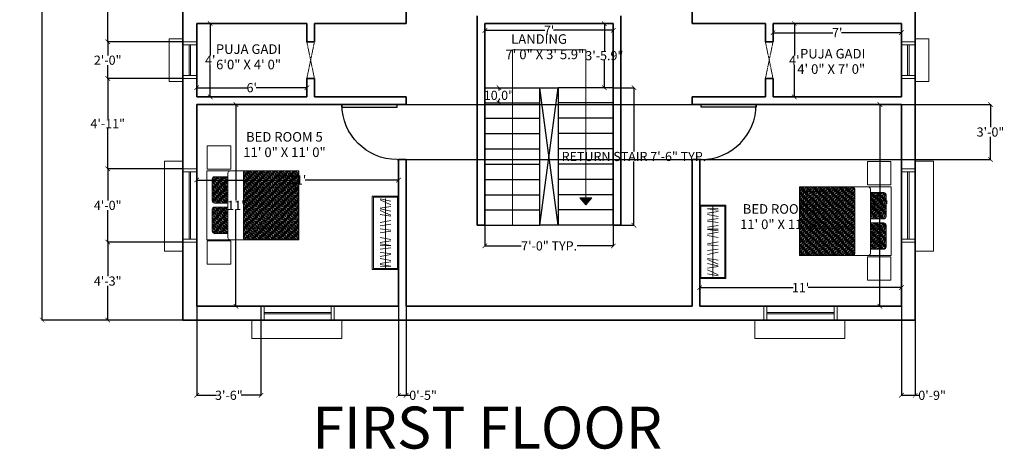
# Model space of a CAD drawing. Units: inches. Extents: x 844 to 2234, y 346 to 1084.
# Tile 47 of 93: x 1590 to 2234, y 351 to 632. Entities that reach past the tile are written whole.
import ezdxf

# ---------------------------------------------------------------- set-up
doc = ezdxf.new("R2010")
doc.units = ezdxf.units.IN
doc.header["$MEASUREMENT"] = 0
doc.linetypes.add('DASHED', pattern=[0.75, 0.5, -0.25])
for name, color, linetype, lineweight in [('A-ANNO-DIMS', 2, 'Continuous', 18), ('A-ANNO-SYMB', 7, 'Continuous', 18), ('A-ANNO-TEXT', 7, 'Continuous', 35), ('A-AREA-IDEN', 7, 'Continuous', 18), ('A-FLOR-STRS', 7, 'Continuous', 25), ('A-WALL', 7, 'Continuous', 35), ('A-WALL-OVHD', 7, 'DASHED', 18), ('beds', 130, 'Continuous', 18), ('doors', 170, 'Continuous', 25), ('furniture', 8, 'Continuous', 18), ('windows', 1, 'Continuous', 18)]:
    doc.layers.add(name, color=color, linetype=linetype, lineweight=lineweight)
doc.styles.get("Standard").update_dxf_attribs({"font": 'arial.ttf'})
doc.dimstyles.get("Standard").update_dxf_attribs({"dimtxt": 6, "dimasz": 3, "dimexe": 0.18, "dimexo": 0.0625, "dimgap": 0.09, "dimtad": 0, "dimtih": 1, "dimtoh": 1, "dimdec": 1, "dimzin": 0, "dimdsep": 46, "dimlunit": 3, "dimtxsty": 'Standard', "dimblk": 'ARCHTICK', "dimcen": 0.09, "dimadec": 0, "dimazin": 0, "dimtfac": 1, "dimtdec": 1, "dimtofl": 0, "dimtmove": 0, "dimatfit": 3, "dimfxl": 1, "dimtolj": 1, "dimtzin": 0, "dimarcsym": 0})
pattern_1 = [(135, (-1377.70473, -125.71507), (-0.070710678, -0.070710678), []), (135, (-1377.68705, -125.69739), (-0.070710678, -0.070710678), []), (45, (-1377.70473, -125.71507), (-0.070710678, 0.070710678), [-0.025, 0.025]), (45, (-1377.72241, -125.69739), (-0.070710678, 0.070710678), [-0.025, 0.025]), (45, (-1377.74009, -125.67972), (-0.070710678, 0.070710678), [0.025, -0.025]), (45, (-1377.75776, -125.66204), (-0.070710678, 0.070710678), [0.025, -0.025]), (135, (-1377.66938, -125.67972), (-0.070710678, -0.070710678), [0.025, -0.025]), (135, (-1377.6517, -125.66204), (-0.070710678, -0.070710678), [0.025, -0.025])]

# ---------------------------------------------------------------- blocks, each defined once
blk = doc.blocks.new('*U2')
for p, q in [((0, 0), (0, -6)), ((36, 0), (36, -6))]:
    blk.add_line(p, q)
blk.add_lwpolyline([(0, 0), (0, 36), (1.75, 36), (1.75, 0)], close=True)
blk.add_arc((0, 0), 36, 0, 90)
blk = doc.blocks.new('MAT-P10')
h = blk.add_hatch()
h.set_pattern_fill('BOX', color=256, scale=0.1, angle=45, style=0)
h.set_pattern_definition(pattern_1)
h.paths.add_polyline_path([(-0.157, 1.46), (0.417, 1.46), (0.417, 1.751, 0.414214), (0.367, 1.801), (-0.107, 1.801, 0.414214), (-0.157, 1.751)])
h.paths.add_polyline_path([(0.505, 1.46), (1.079, 1.46), (1.079, 1.751, 0.414214), (1.029, 1.801), (0.555, 1.801, 0.414214), (0.505, 1.751)])
h = blk.add_hatch()
h.set_pattern_fill('BOX', color=256, scale=0.1, angle=45, style=0)
h.set_pattern_definition(pattern_1)
edge = h.paths.add_edge_path()
edge.add_line((1.205, -0.085), (1.205, 1.062))
edge.add_ellipse((1.161, 1.063), major_axis=(0, 0.0568), ratio=0.776379, start_angle=270, end_angle=360)
edge.add_line((1.161, 1.119), (-0.251, 1.12))
edge.add_ellipse((-0.251, 1.063), major_axis=(0, 0.0568), ratio=0.776379, start_angle=0, end_angle=88.1396)
edge.add_line((-0.295, 1.064), (-0.295, -0.085))
edge.add_line((-0.295, -0.085), (1.205, -0.085))
for p, q in [((-0.251, 1.46), (1.161, 1.46)), ((-0.251, 1.12), (1.161, 1.119)), ((1.102, 0.406), (1.102, 0.057)), ((1.058, 0), (0.775, 0))]:
    blk.add_line(p, q)
for points in [[(-0.83, 1.909), (-0.319, 1.909), (-0.319, 1.398), (-0.83, 1.398)], [(1.205, -0.085), (-0.295, -0.085), (-0.295, 1.915), (1.205, 1.915)], [(1.244, 1.909), (1.755, 1.909), (1.755, 1.398), (1.244, 1.398)]]:
    blk.add_lwpolyline(points, close=True)
for points in [[(0.417, 1.46), (0.417, 1.751, 0.414214), (0.367, 1.801), (-0.107, 1.801, 0.414214), (-0.157, 1.751), (-0.157, 1.46)], [(1.079, 1.46), (1.079, 1.751, 0.414214), (1.029, 1.801), (0.555, 1.801, 0.414214), (0.505, 1.751), (0.505, 1.46)], [(0.37, 1.624), (0.37, 1.571, -0.414214), (0.32, 1.521), (0.111, 1.521)], [(1.012, 1.644), (1.012, 1.571, -0.414214), (0.962, 1.521), (0.753, 1.521)]]:
    blk.add_lwpolyline(points, format="xyb")
at = {"extrusion": (0, 0, -1)}
for centre, start_param, end_param in [((-0.251, 1.404), 4.712389, 6.283185), ((1.161, 1.404), 0, 1.570796), ((-0.251, 1.063), 4.712389, 6.283185), ((1.161, 1.063), 0, 1.570796), ((1.058, 0.057), 1.570796, 3.141593), ((1.058, 0.057), 1.570796, 3.141593)]:
    blk.add_ellipse(centre, major_axis=(0, 0.0568), ratio=0.776379, start_param=start_param, end_param=end_param, dxfattribs=at)
blk = doc.blocks.new('A$C7A17768A')
for p, q in [((-2.8, 0), (0, 0)), ((-2.8, -1), (-2.8, 0)), ((0, -1), (0, 0)), ((-2.76, -0.04), (-0.04, -0.04)), ((-2.76, -0.96), (-2.76, -0.04)), ((-2.617, -0.3), (-2.694, -0.7)), ((-2.66, -0.7), (-2.466, -0.3)), ((-2.403, -0.3), (-2.342, -0.7)), ((-2.229, -0.296), (-2.317, -0.696)), ((-2.074, -0.3), (-2.25, -0.7)), ((-2.096, -0.7), (-2.033, -0.3)), ((-1.875, -0.3), (-1.796, -0.7)), ((-1.732, -0.3), (-1.675, -0.7)), ((-1.555, -0.7), (-1.507, -0.3)), ((-1.467, -0.3), (-1.403, -0.7)), ((-1.227, -0.7), (-1.151, -0.3)), ((-1.098, -0.3), (-1.034, -0.7)), ((-0.98, -0.7), (-0.921, -0.3)), ((-0.908, -0.3), (-0.919, -0.7)), ((-0.834, -0.3), (-0.777, -0.7)), ((-0.657, -0.7), (-0.61, -0.3)), ((-0.57, -0.3), (-0.505, -0.7)), ((-0.429, -0.7), (-0.353, -0.3)), ((-0.301, -0.3), (-0.237, -0.7)), ((-0.192, -0.7), (-0.133, -0.3)), ((-0.12, -0.3), (-0.131, -0.7)), ((-0.04, -0.96), (-0.04, -0.04)), ((-0.04, -0.5), (-2.716, -0.5)), ((-2.8, -1), (0, -1)), ((-2.76, -0.96), (-0.04, -0.96))]:
    blk.add_line(p, q)
blk = doc.blocks.new('_ArchTick')
at = {"color": 0, "linetype": 'ByBlock', "const_width": 0.15}
blk.add_lwpolyline([(-0.5, -0.5), (0.5, 0.5)], dxfattribs=at)
blk = doc.blocks.new('*D69')
at = {"layer": 'A-ANNO-DIMS', "color": 0, "lineweight": -2, "transparency": 16777216}
for p, q in [((2125.04, 629.46), (2096.85, 629.46)), ((2097.03, 629.46), (2097.03, 608.55)), ((2097.03, 581.46), (2097.03, 602.37)), ((2125.04, 581.46), (2096.85, 581.46))]:
    blk.add_line(p, q, dxfattribs=at)
at = {"layer": 'Defpoints', "color": 0, "transparency": 16777216}
for p in [(2125.1, 629.46), (2097.03, 581.46), (2125.1, 581.46)]:
    blk.add_point(p, dxfattribs=at)
at = {"layer": 'A-ANNO-DIMS', "color": 0, "lineweight": -2, "transparency": 16777216, "xscale": 3, "yscale": 3, "zscale": 3}
for p, rotation in [((2097.03, 629.46), 90), ((2097.03, 581.46), 270)]:
    blk.add_blockref('_ArchTick', p, dxfattribs=dict(at, rotation=rotation))
at = {"layer": 'A-ANNO-DIMS', "color": 0, "transparency": 16777216, "insert": (2097.03, 605.46), "char_height": 6, "attachment_point": 5}
blk.add_mtext("\\A1;4'", dxfattribs=at)
blk = doc.blocks.new('*D70')
at = {"layer": 'A-ANNO-DIMS', "color": 0, "lineweight": -2, "transparency": 16777216}
for p, q in [((2083.1, 623.52), (2083.1, 623.64)), ((2083.1, 623.46), (2122.27, 623.46)), ((2167.1, 623.46), (2127.93, 623.46)), ((2167.1, 623.52), (2167.1, 623.64))]:
    blk.add_line(p, q, dxfattribs=at)
at = {"layer": 'Defpoints', "color": 0, "transparency": 16777216}
for p in [(2083.1, 623.46), (2167.1, 623.46), (2167.1, 623.46)]:
    blk.add_point(p, dxfattribs=at)
at = {"layer": 'A-ANNO-DIMS', "color": 0, "lineweight": -2, "transparency": 16777216, "xscale": 3, "yscale": 3, "zscale": 3, "rotation": 180}
blk.add_blockref('_ArchTick', (2083.1, 623.46), dxfattribs=at)
at = {"layer": 'A-ANNO-DIMS', "color": 0, "lineweight": -2, "transparency": 16777216, "xscale": 3, "yscale": 3, "zscale": 3}
blk.add_blockref('_ArchTick', (2167.1, 623.46), dxfattribs=at)
at = {"layer": 'A-ANNO-DIMS', "color": 0, "transparency": 16777216, "insert": (2125.1, 623.46), "char_height": 6, "attachment_point": 5}
blk.add_mtext("\\A1;7'", dxfattribs=at)
blk = doc.blocks.new('*D61')
at = {"layer": 'A-ANNO-DIMS', "color": 0, "lineweight": -2, "transparency": 16777216}
for p, q in [((1706.1, 585.7), (1706.1, 587.64)), ((1706.1, 587.46), (1739.23, 587.46)), ((1778.1, 587.46), (1744.97, 587.46)), ((1778.1, 585.7), (1778.1, 587.64))]:
    blk.add_line(p, q, dxfattribs=at)
at = {"layer": 'Defpoints', "color": 0, "transparency": 16777216}
for p in [(1778.1, 587.46), (1706.1, 585.64), (1778.1, 585.64)]:
    blk.add_point(p, dxfattribs=at)
at = {"layer": 'A-ANNO-DIMS', "color": 0, "lineweight": -2, "transparency": 16777216, "xscale": 3, "yscale": 3, "zscale": 3, "rotation": 180}
blk.add_blockref('_ArchTick', (1706.1, 587.46), dxfattribs=at)
at = {"layer": 'A-ANNO-DIMS', "color": 0, "lineweight": -2, "transparency": 16777216, "xscale": 3, "yscale": 3, "zscale": 3}
blk.add_blockref('_ArchTick', (1778.1, 587.46), dxfattribs=at)
at = {"layer": 'A-ANNO-DIMS', "color": 0, "transparency": 16777216, "insert": (1742.1, 587.46), "char_height": 6, "attachment_point": 5}
blk.add_mtext("\\A1;6'", dxfattribs=at)
blk = doc.blocks.new('*D62')
at = {"layer": 'A-ANNO-DIMS', "color": 0, "lineweight": -2, "transparency": 16777216}
for p, q in [((1715.1, 629.46), (1714.74, 629.46)), ((1714.92, 629.46), (1714.92, 608.55)), ((1714.92, 581.46), (1714.92, 602.37)), ((1715.1, 581.46), (1714.74, 581.46))]:
    blk.add_line(p, q, dxfattribs=at)
at = {"layer": 'Defpoints', "color": 0, "transparency": 16777216}
for p in [(1715.17, 629.46), (1714.92, 581.46), (1715.17, 581.46)]:
    blk.add_point(p, dxfattribs=at)
at = {"layer": 'A-ANNO-DIMS', "color": 0, "lineweight": -2, "transparency": 16777216, "xscale": 3, "yscale": 3, "zscale": 3}
for p, rotation in [((1714.92, 629.46), 90), ((1714.92, 581.46), 270)]:
    blk.add_blockref('_ArchTick', p, dxfattribs=dict(at, rotation=rotation))
at = {"layer": 'A-ANNO-DIMS', "color": 0, "transparency": 16777216, "insert": (1714.92, 605.46), "char_height": 6, "attachment_point": 5}
blk.add_mtext("\\A1;4'", dxfattribs=at)
blk = doc.blocks.new('*D76')
at = {"layer": 'A-ANNO-DIMS', "color": 0, "lineweight": -2, "transparency": 16777216}
for p, q in [((1711.63, 576.46), (1731.95, 576.46)), ((1731.77, 576.46), (1731.77, 513.56)), ((1731.77, 444.46), (1731.77, 507.35)), ((1711.63, 444.46), (1731.95, 444.46))]:
    blk.add_line(p, q, dxfattribs=at)
at = {"layer": 'Defpoints', "color": 0, "transparency": 16777216}
for p in [(1711.57, 576.46), (1711.57, 444.46), (1731.77, 444.46)]:
    blk.add_point(p, dxfattribs=at)
at = {"layer": 'A-ANNO-DIMS', "color": 0, "lineweight": -2, "transparency": 16777216, "xscale": 3, "yscale": 3, "zscale": 3}
for p, rotation in [((1731.77, 576.46), 90), ((1731.77, 444.46), 270)]:
    blk.add_blockref('_ArchTick', p, dxfattribs=dict(at, rotation=rotation))
at = {"layer": 'A-ANNO-DIMS', "color": 0, "transparency": 16777216, "insert": (1731.77, 510.46), "char_height": 6, "attachment_point": 5}
blk.add_mtext("\\A1;11'", dxfattribs=at)
blk = doc.blocks.new('*D77')
at = {"layer": 'A-ANNO-DIMS', "color": 0, "lineweight": -2, "transparency": 16777216}
for p, q in [((1706.1, 526.13), (1706.1, 527.23)), ((1706.1, 527.05), (1767.2, 527.05)), ((1838.1, 527.05), (1777, 527.05)), ((1838.1, 526.13), (1838.1, 527.23))]:
    blk.add_line(p, q, dxfattribs=at)
at = {"layer": 'Defpoints', "color": 0, "transparency": 16777216}
for p in [(1706.1, 527.05), (1706.1, 526.07), (1838.1, 526.07)]:
    blk.add_point(p, dxfattribs=at)
at = {"layer": 'A-ANNO-DIMS', "color": 0, "lineweight": -2, "transparency": 16777216, "xscale": 3, "yscale": 3, "zscale": 3, "rotation": 180}
blk.add_blockref('_ArchTick', (1706.1, 527.05), dxfattribs=at)
at = {"layer": 'A-ANNO-DIMS', "color": 0, "lineweight": -2, "transparency": 16777216, "xscale": 3, "yscale": 3, "zscale": 3}
blk.add_blockref('_ArchTick', (1838.1, 527.05), dxfattribs=at)
at = {"layer": 'A-ANNO-DIMS', "color": 0, "transparency": 16777216, "insert": (1772.1, 527.05), "char_height": 6, "attachment_point": 5}
blk.add_mtext("\\A1;11'", dxfattribs=at)
blk = doc.blocks.new('*D78')
at = {"layer": 'A-ANNO-DIMS', "color": 0, "lineweight": -2, "transparency": 16777216}
for p, q in [((2035.1, 454.11), (2035.1, 456.83)), ((2035.1, 456.65), (2096.2, 456.65)), ((2167.1, 456.65), (2106, 456.65)), ((2167.1, 454.11), (2167.1, 456.83))]:
    blk.add_line(p, q, dxfattribs=at)
at = {"layer": 'Defpoints', "color": 0, "transparency": 16777216}
for p in [(2035.1, 454.05), (2167.1, 456.65), (2167.1, 454.05)]:
    blk.add_point(p, dxfattribs=at)
at = {"layer": 'A-ANNO-DIMS', "color": 0, "lineweight": -2, "transparency": 16777216, "xscale": 3, "yscale": 3, "zscale": 3, "rotation": 180}
blk.add_blockref('_ArchTick', (2035.1, 456.65), dxfattribs=at)
at = {"layer": 'A-ANNO-DIMS', "color": 0, "lineweight": -2, "transparency": 16777216, "xscale": 3, "yscale": 3, "zscale": 3}
blk.add_blockref('_ArchTick', (2167.1, 456.65), dxfattribs=at)
at = {"layer": 'A-ANNO-DIMS', "color": 0, "transparency": 16777216, "insert": (2101.1, 456.65), "char_height": 6, "attachment_point": 5}
blk.add_mtext("\\A1;11'", dxfattribs=at)
blk = doc.blocks.new('*D79')
at = {"layer": 'A-ANNO-DIMS', "color": 0, "lineweight": -2, "transparency": 16777216}
for p, q in [((2156.99, 576.46), (2152.84, 576.46)), ((2153.02, 576.46), (2153.02, 513.56)), ((2153.02, 444.46), (2153.02, 507.35)), ((2156.99, 444.46), (2152.84, 444.46))]:
    blk.add_line(p, q, dxfattribs=at)
at = {"layer": 'Defpoints', "color": 0, "transparency": 16777216}
for p in [(2157.05, 576.46), (2153.02, 444.46), (2157.05, 444.46)]:
    blk.add_point(p, dxfattribs=at)
at = {"layer": 'A-ANNO-DIMS', "color": 0, "lineweight": -2, "transparency": 16777216, "xscale": 3, "yscale": 3, "zscale": 3}
for p, rotation in [((2153.02, 576.46), 90), ((2153.02, 444.46), 270)]:
    blk.add_blockref('_ArchTick', p, dxfattribs=dict(at, rotation=rotation))
at = {"layer": 'A-ANNO-DIMS', "color": 0, "transparency": 16777216, "insert": (2153.02, 510.46), "char_height": 6, "attachment_point": 5}
blk.add_mtext("\\A1;11'", dxfattribs=at)
blk = doc.blocks.new('*D81')
at = {"layer": 'A-ANNO-DIMS', "color": 0, "lineweight": -2, "transparency": 16777216}
for p, q in [((1903.27, 587.46), (1903.94, 587.46)), ((1903.76, 587.46), (1903.76, 585.61)), ((1903.27, 577.46), (1903.94, 577.46)), ((1903.76, 577.46), (1903.76, 579.3))]:
    blk.add_line(p, q, dxfattribs=at)
at = {"layer": 'Defpoints', "color": 0, "transparency": 16777216}
for p in [(1903.21, 587.46), (1903.21, 577.46), (1903.76, 577.46)]:
    blk.add_point(p, dxfattribs=at)
at = {"layer": 'A-ANNO-DIMS', "color": 0, "lineweight": -2, "transparency": 16777216, "xscale": 3, "yscale": 3, "zscale": 3}
for p, rotation in [((1903.76, 587.46), 90), ((1903.76, 577.46), 270)]:
    blk.add_blockref('_ArchTick', p, dxfattribs=dict(at, rotation=rotation))
at = {"layer": 'A-ANNO-DIMS', "color": 0, "transparency": 16777216, "insert": (1903.76, 582.46), "char_height": 6, "attachment_point": 5}
blk.add_mtext('\\A1;10.0"', dxfattribs=at)
blk = doc.blocks.new('*D82')
at = {"layer": 'A-ANNO-DIMS', "color": 0, "lineweight": -2, "transparency": 16777216}
for p, q in [((1894.6, 625.06), (1894.6, 625.18)), ((1894.6, 625), (1933.77, 625)), ((1978.6, 625), (1939.43, 625)), ((1978.6, 625.06), (1978.6, 625.18))]:
    blk.add_line(p, q, dxfattribs=at)
at = {"layer": 'Defpoints', "color": 0, "transparency": 16777216}
for p in [(1894.6, 625), (1978.6, 625), (1978.6, 625)]:
    blk.add_point(p, dxfattribs=at)
at = {"layer": 'A-ANNO-DIMS', "color": 0, "lineweight": -2, "transparency": 16777216, "xscale": 3, "yscale": 3, "zscale": 3, "rotation": 180}
blk.add_blockref('_ArchTick', (1894.6, 625), dxfattribs=at)
at = {"layer": 'A-ANNO-DIMS', "color": 0, "lineweight": -2, "transparency": 16777216, "xscale": 3, "yscale": 3, "zscale": 3}
blk.add_blockref('_ArchTick', (1978.6, 625), dxfattribs=at)
at = {"layer": 'A-ANNO-DIMS', "color": 0, "transparency": 16777216, "insert": (1936.6, 625), "char_height": 6, "attachment_point": 5}
blk.add_mtext("\\A1;7'", dxfattribs=at)
blk = doc.blocks.new('*D83')
at = {"layer": 'A-ANNO-DIMS', "color": 0, "lineweight": -2, "transparency": 16777216}
for p, q in [((1972.71, 629.39), (1972.92, 629.39)), ((1972.74, 629.39), (1972.74, 611.58)), ((1972.74, 587.46), (1972.74, 605.27)), ((1972.71, 587.46), (1972.92, 587.46))]:
    blk.add_line(p, q, dxfattribs=at)
at = {"layer": 'Defpoints', "color": 0, "transparency": 16777216}
for p in [(1972.65, 629.39), (1972.65, 587.46), (1972.74, 587.46)]:
    blk.add_point(p, dxfattribs=at)
at = {"layer": 'A-ANNO-DIMS', "color": 0, "lineweight": -2, "transparency": 16777216, "xscale": 3, "yscale": 3, "zscale": 3}
for p, rotation in [((1972.74, 629.39), 90), ((1972.74, 587.46), 270)]:
    blk.add_blockref('_ArchTick', p, dxfattribs=dict(at, rotation=rotation))
at = {"layer": 'A-ANNO-DIMS', "color": 0, "transparency": 16777216, "insert": (1972.74, 608.43), "char_height": 6, "attachment_point": 5}
blk.add_mtext('\\A1;3\'-5.9"', dxfattribs=at)
blk = doc.blocks.new('*D87')
at = {"layer": 'A-ANNO-DIMS', "color": 0, "lineweight": -2, "transparency": 16777216}
for p, q in [((1697.04, 1030.46), (1604.81, 1030.46)), ((1604.99, 1030.46), (1604.99, 736.11)), ((1604.99, 435.46), (1604.99, 729.8)), ((1697.04, 435.46), (1604.81, 435.46))]:
    blk.add_line(p, q, dxfattribs=at)
at = {"layer": 'Defpoints', "color": 0, "transparency": 16777216}
for p in [(1697.1, 1030.46), (1604.99, 435.46), (1697.1, 435.46)]:
    blk.add_point(p, dxfattribs=at)
at = {"layer": 'A-ANNO-DIMS', "color": 0, "lineweight": -2, "transparency": 16777216, "xscale": 3, "yscale": 3, "zscale": 3}
for p, rotation in [((1604.99, 1030.46), 90), ((1604.99, 435.46), 270)]:
    blk.add_blockref('_ArchTick', p, dxfattribs=dict(at, rotation=rotation))
at = {"layer": 'A-ANNO-DIMS', "color": 0, "transparency": 16777216, "insert": (1604.99, 732.96), "char_height": 6, "attachment_point": 5}
blk.add_mtext('\\A1;49\'-7.0"', dxfattribs=at)
blk = doc.blocks.new('WIN-48IN')
for p, q in [((0, 9), (0, 21)), ((0, 21), (59, 21)), ((59, 9), (59, 21)), ((6, 9), (0, 9)), ((54, 9), (6, 9)), ((6, 9), (6, 0)), ((8, 9), (8, 0)), ((52, 0), (52, 9)), ((54, 0), (54, 9)), ((54, 9), (59, 9)), ((8, 5), (52, 5)), ((8, 4), (52, 4)), ((6, 0), (54, 0))]:
    blk.add_line(p, q)
blk = doc.blocks.new('WIN-24IN')
for p, q in [((9, 28), (0, 28)), ((0, 0), (0, 28)), ((9, 26), (9, 28)), ((18, 26), (9, 26)), ((9, 26), (9, 2)), ((18, 2), (18, 26)), ((18, 24), (9, 24)), ((13, 4), (13, 24)), ((14, 4), (14, 24)), ((9, 4), (18, 4)), ((9, 2), (18, 2)), ((9, 2), (9, 0)), ((9, 0), (0, 0))]:
    blk.add_line(p, q)
blk = doc.blocks.new('STAIR-RETURN-FLIGHTS')
for p, q in [((0, 90), (36, 90)), ((36, 0), (36, 90)), ((36, 90), (48, 90)), ((48, 0), (36, 90)), ((36, 0), (48, 90)), ((84, 90), (48, 90)), ((48, 90), (48, 0)), ((0, 80), (36, 80)), ((84, 80), (48, 80)), ((0, 70), (36, 70)), ((84, 70), (48, 70)), ((0, 60), (36, 60)), ((84, 60), (48, 60)), ((0, 50), (36, 50)), ((84, 50), (48, 50)), ((0, 40), (36, 40)), ((84, 40), (48, 40)), ((0, 30), (36, 30)), ((84, 30), (48, 30)), ((0, 20), (36, 20)), ((84, 20), (48, 20)), ((0, 10), (36, 10)), ((84, 10), (48, 10)), ((0, 0), (36, 0)), ((48, 0), (36, 0)), ((84, 0), (48, 0))]:
    blk.add_line(p, q)
blk = doc.blocks.new('STAIR-DIRECTION-RETURN')
h = blk.add_hatch(color=256)
h.dxf.hatch_style = 1
h.paths.add_polyline_path([(52, 17.85), (48, 17.85), (44, 17.85), (48, 13.33)])
for p, q in [((0, 0), (0, 114.78)), ((0, 114.78), (48, 114.78)), ((48, 114.78), (48, 17.85)), ((48, 17.85), (44, 17.85)), ((48, 13.33), (44, 17.85)), ((48, 17.85), (52, 17.85)), ((52, 17.85), (48, 13.33))]:
    blk.add_line(p, q)
blk = doc.blocks.new('*D139')
at = {"layer": 'A-ANNO-DIMS', "color": 0, "lineweight": -2, "transparency": 16777216}
for p, q in [((1978.66, 587.46), (1992.28, 587.46)), ((1992.1, 587.46), (1992.1, 545.65)), ((1992.1, 497.46), (1992.1, 539.26)), ((1978.66, 497.46), (1992.28, 497.46))]:
    blk.add_line(p, q, dxfattribs=at)
at = {"layer": 'Defpoints', "color": 0, "transparency": 16777216}
for p in [(1978.6, 587.46), (1992.1, 587.46), (1978.6, 497.46)]:
    blk.add_point(p, dxfattribs=at)
at = {"layer": 'A-ANNO-DIMS', "color": 0, "lineweight": -2, "transparency": 16777216, "xscale": 3, "yscale": 3, "zscale": 3}
for p, rotation in [((1992.1, 587.46), 90), ((1992.1, 497.46), 270)]:
    blk.add_blockref('_ArchTick', p, dxfattribs=dict(at, rotation=rotation))
at = {"layer": 'A-ANNO-DIMS', "color": 0, "transparency": 16777216, "insert": (1992.1, 542.46), "char_height": 6, "attachment_point": 5}
blk.add_mtext('\\A1;RETURN STAIR 7\'-6" TYP.', dxfattribs=at)
blk = doc.blocks.new('*D140')
at = {"layer": 'A-ANNO-DIMS', "color": 0, "lineweight": -2, "transparency": 16777216}
for p, q in [((1894.6, 497.39), (1894.6, 483.78)), ((1978.6, 497.39), (1978.6, 483.78)), ((1894.6, 483.96), (1918.25, 483.96)), ((1978.6, 483.96), (1954.95, 483.96))]:
    blk.add_line(p, q, dxfattribs=at)
at = {"layer": 'Defpoints', "color": 0, "transparency": 16777216}
for p in [(1894.6, 497.46), (1978.6, 497.46), (1978.6, 483.96)]:
    blk.add_point(p, dxfattribs=at)
at = {"layer": 'A-ANNO-DIMS', "color": 0, "lineweight": -2, "transparency": 16777216, "xscale": 3, "yscale": 3, "zscale": 3, "rotation": 180}
blk.add_blockref('_ArchTick', (1894.6, 483.96), dxfattribs=at)
at = {"layer": 'A-ANNO-DIMS', "color": 0, "lineweight": -2, "transparency": 16777216, "xscale": 3, "yscale": 3, "zscale": 3}
blk.add_blockref('_ArchTick', (1978.6, 483.96), dxfattribs=at)
at = {"layer": 'A-ANNO-DIMS', "color": 0, "transparency": 16777216, "insert": (1936.6, 483.96), "char_height": 6, "attachment_point": 5}
blk.add_mtext('\\A1;7\'-0" TYP.', dxfattribs=at)
blk = doc.blocks.new('*D145')
at = {"layer": 'A-ANNO-DIMS', "color": 0, "lineweight": -2, "transparency": 16777216}
for p, q in [((1838.1, 444.39), (1838.1, 386.03)), ((1843.1, 444.39), (1843.1, 386.03)), ((1838.1, 386.21), (1843.1, 386.21)), ((1843.1, 386.21), (1846.1, 386.21))]:
    blk.add_line(p, q, dxfattribs=at)
at = {"layer": 'Defpoints', "color": 0, "transparency": 16777216}
for p in [(1838.1, 444.46), (1843.1, 444.46), (1843.1, 386.21)]:
    blk.add_point(p, dxfattribs=at)
at = {"layer": 'A-ANNO-DIMS', "color": 0, "lineweight": -2, "transparency": 16777216, "xscale": 3, "yscale": 3, "zscale": 3, "rotation": 180}
blk.add_blockref('_ArchTick', (1838.1, 386.21), dxfattribs=at)
at = {"layer": 'A-ANNO-DIMS', "color": 0, "lineweight": -2, "transparency": 16777216, "xscale": 3, "yscale": 3, "zscale": 3}
blk.add_blockref('_ArchTick', (1843.1, 386.21), dxfattribs=at)
at = {"layer": 'A-ANNO-DIMS', "color": 0, "transparency": 16777216, "insert": (1854.16, 386.21), "char_height": 6, "attachment_point": 5}
blk.add_mtext('\\A1;0\'-5"', dxfattribs=at)
blk = doc.blocks.new('*D146')
at = {"layer": 'A-ANNO-DIMS', "color": 0, "lineweight": -2, "transparency": 16777216}
for p, q in [((2167.1, 444.39), (2167.1, 386.03)), ((2176.1, 435.39), (2176.1, 386.03)), ((2167.1, 386.21), (2176.1, 386.21)), ((2176.1, 386.21), (2179.1, 386.21))]:
    blk.add_line(p, q, dxfattribs=at)
at = {"layer": 'Defpoints', "color": 0, "transparency": 16777216}
for p in [(2167.1, 444.46), (2176.1, 435.46), (2176.1, 386.21)]:
    blk.add_point(p, dxfattribs=at)
at = {"layer": 'A-ANNO-DIMS', "color": 0, "lineweight": -2, "transparency": 16777216, "xscale": 3, "yscale": 3, "zscale": 3, "rotation": 180}
blk.add_blockref('_ArchTick', (2167.1, 386.21), dxfattribs=at)
at = {"layer": 'A-ANNO-DIMS', "color": 0, "lineweight": -2, "transparency": 16777216, "xscale": 3, "yscale": 3, "zscale": 3}
blk.add_blockref('_ArchTick', (2176.1, 386.21), dxfattribs=at)
at = {"layer": 'A-ANNO-DIMS', "color": 0, "transparency": 16777216, "insert": (2187.16, 386.21), "char_height": 6, "attachment_point": 5}
blk.add_mtext('\\A1;0\'-9"', dxfattribs=at)
blk = doc.blocks.new('*D147')
at = {"layer": 'A-ANNO-DIMS', "color": 0, "lineweight": -2, "transparency": 16777216}
for p, q in [((1706.1, 444.39), (1706.1, 386.03)), ((1748.1, 444.39), (1748.1, 386.03)), ((1706.1, 386.21), (1719.04, 386.21)), ((1748.1, 386.21), (1735.16, 386.21))]:
    blk.add_line(p, q, dxfattribs=at)
at = {"layer": 'Defpoints', "color": 0, "transparency": 16777216}
for p in [(1706.1, 444.46), (1748.1, 444.46), (1748.1, 386.21)]:
    blk.add_point(p, dxfattribs=at)
at = {"layer": 'A-ANNO-DIMS', "color": 0, "lineweight": -2, "transparency": 16777216, "xscale": 3, "yscale": 3, "zscale": 3, "rotation": 180}
blk.add_blockref('_ArchTick', (1706.1, 386.21), dxfattribs=at)
at = {"layer": 'A-ANNO-DIMS', "color": 0, "lineweight": -2, "transparency": 16777216, "xscale": 3, "yscale": 3, "zscale": 3}
blk.add_blockref('_ArchTick', (1748.1, 386.21), dxfattribs=at)
at = {"layer": 'A-ANNO-DIMS', "color": 0, "transparency": 16777216, "insert": (1727.1, 386.21), "char_height": 6, "attachment_point": 5}
blk.add_mtext('\\A1;3\'-6"', dxfattribs=at)
blk = doc.blocks.new('*D148')
at = {"layer": 'A-ANNO-DIMS', "color": 0, "lineweight": -2, "transparency": 16777216}
for p, q in [((1838.16, 576.46), (2225.53, 576.46)), ((2225.35, 576.46), (2225.35, 561.61)), ((2225.35, 540.46), (2225.35, 555.3)), ((1838.16, 540.46), (2225.53, 540.46))]:
    blk.add_line(p, q, dxfattribs=at)
at = {"layer": 'Defpoints', "color": 0, "transparency": 16777216}
for p in [(1838.1, 576.46), (1838.1, 540.46), (2225.35, 540.46)]:
    blk.add_point(p, dxfattribs=at)
at = {"layer": 'A-ANNO-DIMS', "color": 0, "lineweight": -2, "transparency": 16777216, "xscale": 3, "yscale": 3, "zscale": 3}
for p, rotation in [((2225.35, 576.46), 90), ((2225.35, 540.46), 270)]:
    blk.add_blockref('_ArchTick', p, dxfattribs=dict(at, rotation=rotation))
at = {"layer": 'A-ANNO-DIMS', "color": 0, "transparency": 16777216, "insert": (2225.35, 558.46), "char_height": 6, "attachment_point": 5}
blk.add_mtext('\\A1;3\'-0"', dxfattribs=at)
blk = doc.blocks.new('*D159')
at = {"layer": 'A-ANNO-DIMS', "color": 0, "lineweight": -2, "transparency": 16777216}
for p, q in [((1697.04, 486.46), (1647.67, 486.46)), ((1647.85, 486.46), (1647.85, 464.11)), ((1647.85, 435.46), (1647.85, 457.8)), ((1697.04, 435.46), (1647.67, 435.46))]:
    blk.add_line(p, q, dxfattribs=at)
at = {"layer": 'Defpoints', "color": 0, "transparency": 16777216}
for p in [(1647.85, 486.46), (1697.1, 486.46), (1697.1, 435.46)]:
    blk.add_point(p, dxfattribs=at)
at = {"layer": 'A-ANNO-DIMS', "color": 0, "lineweight": -2, "transparency": 16777216, "xscale": 3, "yscale": 3, "zscale": 3}
for p, rotation in [((1647.85, 486.46), 90), ((1647.85, 435.46), 270)]:
    blk.add_blockref('_ArchTick', p, dxfattribs=dict(at, rotation=rotation))
at = {"layer": 'A-ANNO-DIMS', "color": 0, "transparency": 16777216, "insert": (1647.85, 460.96), "char_height": 6, "attachment_point": 5}
blk.add_mtext('\\A1;4\'-3"', dxfattribs=at)
blk = doc.blocks.new('*D160')
at = {"layer": 'A-ANNO-DIMS', "color": 0, "lineweight": -2, "transparency": 16777216}
for p, q in [((1697.04, 534.46), (1647.67, 534.46)), ((1647.85, 534.46), (1647.85, 513.61)), ((1647.85, 486.46), (1647.85, 507.3)), ((1697.04, 486.46), (1647.67, 486.46))]:
    blk.add_line(p, q, dxfattribs=at)
at = {"layer": 'Defpoints', "color": 0, "transparency": 16777216}
for p in [(1647.85, 534.46), (1697.1, 534.46), (1697.1, 486.46)]:
    blk.add_point(p, dxfattribs=at)
at = {"layer": 'A-ANNO-DIMS', "color": 0, "lineweight": -2, "transparency": 16777216, "xscale": 3, "yscale": 3, "zscale": 3}
for p, rotation in [((1647.85, 534.46), 90), ((1647.85, 486.46), 270)]:
    blk.add_blockref('_ArchTick', p, dxfattribs=dict(at, rotation=rotation))
at = {"layer": 'A-ANNO-DIMS', "color": 0, "transparency": 16777216, "insert": (1647.85, 510.46), "char_height": 6, "attachment_point": 5}
blk.add_mtext('\\A1;4\'-0"', dxfattribs=at)
blk = doc.blocks.new('*D161')
at = {"layer": 'A-ANNO-DIMS', "color": 0, "lineweight": -2, "transparency": 16777216}
for p, q in [((1697.04, 593.46), (1647.67, 593.46)), ((1647.85, 593.46), (1647.85, 567.06)), ((1647.85, 534.46), (1647.85, 560.85)), ((1697.04, 534.46), (1647.67, 534.46))]:
    blk.add_line(p, q, dxfattribs=at)
at = {"layer": 'Defpoints', "color": 0, "transparency": 16777216}
for p in [(1647.85, 593.46), (1697.1, 593.46), (1697.1, 534.46)]:
    blk.add_point(p, dxfattribs=at)
at = {"layer": 'A-ANNO-DIMS', "color": 0, "lineweight": -2, "transparency": 16777216, "xscale": 3, "yscale": 3, "zscale": 3}
for p, rotation in [((1647.85, 593.46), 90), ((1647.85, 534.46), 270)]:
    blk.add_blockref('_ArchTick', p, dxfattribs=dict(at, rotation=rotation))
at = {"layer": 'A-ANNO-DIMS', "color": 0, "transparency": 16777216, "insert": (1647.85, 563.96), "char_height": 6, "attachment_point": 5}
blk.add_mtext('\\A1;4\'-11"', dxfattribs=at)
blk = doc.blocks.new('*D162')
at = {"layer": 'A-ANNO-DIMS', "color": 0, "lineweight": -2, "transparency": 16777216}
for p, q in [((1697.04, 617.46), (1647.67, 617.46)), ((1647.85, 617.46), (1647.85, 608.61)), ((1647.85, 593.46), (1647.85, 602.3)), ((1697.04, 593.46), (1647.67, 593.46))]:
    blk.add_line(p, q, dxfattribs=at)
at = {"layer": 'Defpoints', "color": 0, "transparency": 16777216}
for p in [(1647.85, 617.46), (1697.1, 617.46), (1697.1, 593.46)]:
    blk.add_point(p, dxfattribs=at)
at = {"layer": 'A-ANNO-DIMS', "color": 0, "lineweight": -2, "transparency": 16777216, "xscale": 3, "yscale": 3, "zscale": 3}
for p, rotation in [((1647.85, 617.46), 90), ((1647.85, 593.46), 270)]:
    blk.add_blockref('_ArchTick', p, dxfattribs=dict(at, rotation=rotation))
at = {"layer": 'A-ANNO-DIMS', "color": 0, "transparency": 16777216, "insert": (1647.85, 605.46), "char_height": 6, "attachment_point": 5}
blk.add_mtext('\\A1;2\'-0"', dxfattribs=at)
blk = doc.blocks.new('*D163')
at = {"layer": 'A-ANNO-DIMS', "color": 0, "lineweight": -2, "transparency": 16777216}
for p, q in [((1697.04, 676.46), (1647.67, 676.46)), ((1647.85, 676.46), (1647.85, 650.06)), ((1647.85, 617.46), (1647.85, 643.85)), ((1697.04, 617.46), (1647.67, 617.46))]:
    blk.add_line(p, q, dxfattribs=at)
at = {"layer": 'Defpoints', "color": 0, "transparency": 16777216}
for p in [(1647.85, 676.46), (1697.1, 676.46), (1697.1, 617.46)]:
    blk.add_point(p, dxfattribs=at)
at = {"layer": 'A-ANNO-DIMS', "color": 0, "lineweight": -2, "transparency": 16777216, "xscale": 3, "yscale": 3, "zscale": 3}
for p, rotation in [((1647.85, 676.46), 90), ((1647.85, 617.46), 270)]:
    blk.add_blockref('_ArchTick', p, dxfattribs=dict(at, rotation=rotation))
at = {"layer": 'A-ANNO-DIMS', "color": 0, "transparency": 16777216, "insert": (1647.85, 646.96), "char_height": 6, "attachment_point": 5}
blk.add_mtext('\\A1;4\'-11"', dxfattribs=at)

msp = doc.modelspace()

# ---------------------------------------------------------------- linework, layer by layer
at = {"layer": 'A-WALL'}
for p, q in [((1697.1, 1030.46), (1697.1, 435.46)), ((2176.1, 1030.46), (2176.1, 435.46)), ((1843.1, 766.46), (1843.1, 629.46)), ((2030.1, 766.46), (2030.1, 629.46)), ((1889.6, 634.46), (1889.6, 521.46)), ((1983.6, 634.46), (1983.6, 521.46)), ((1706.1, 629.46), (1706.1, 581.46)), ((1706.1, 629.46), (1778.1, 629.46)), ((1778.1, 629.46), (1778.1, 617.46)), ((1783.1, 629.46), (1783.1, 617.46)), ((1783.1, 629.46), (1843.1, 629.46)), ((1894.6, 629.46), (1978.6, 629.46)), ((1894.6, 629.46), (1894.6, 521.46)), ((1978.6, 629.46), (1978.6, 521.46)), ((2078.1, 629.46), (2030.1, 629.46)), ((2078.1, 629.46), (2078.1, 617.46)), ((2083.1, 629.46), (2083.1, 617.46)), ((2167.1, 629.46), (2083.1, 629.46)), ((2167.1, 629.46), (2167.1, 581.46)), ((1783.1, 617.46), (1778.1, 617.46)), ((2078.1, 617.46), (2083.1, 617.46)), ((1778.1, 593.46), (1778.1, 581.46)), ((1783.1, 593.46), (1778.1, 593.46)), ((1783.1, 593.46), (1783.1, 581.46)), ((2078.1, 593.46), (2078.1, 581.46)), ((2078.1, 593.46), (2083.1, 593.46)), ((2083.1, 593.46), (2083.1, 581.46)), ((1706.1, 581.46), (1778.1, 581.46)), ((1783.1, 581.46), (1843.1, 581.46)), ((1843.1, 576.46), (1843.1, 581.46)), ((2030.1, 581.46), (2030.1, 576.46)), ((2078.1, 581.46), (2030.1, 581.46)), ((2167.1, 581.46), (2083.1, 581.46)), ((1706.1, 576.46), (1706.1, 444.46)), ((1706.1, 576.46), (1838.1, 576.46)), ((1838.1, 576.46), (1843.1, 576.46)), ((2035.1, 576.46), (2030.1, 576.46)), ((2167.1, 576.46), (2035.1, 576.46)), ((2167.1, 576.46), (2167.1, 444.46)), ((1838.1, 540.46), (1838.1, 444.46)), ((1838.1, 540.46), (1843.1, 540.46)), ((1843.1, 540.46), (1843.1, 444.46)), ((2030.1, 540.46), (2030.1, 444.46)), ((2035.1, 540.46), (2030.1, 540.46)), ((2035.1, 540.46), (2035.1, 444.46)), ((1889.6, 521.46), (1889.6, 497.46)), ((1894.6, 521.46), (1894.6, 497.46)), ((1978.6, 521.46), (1978.6, 497.46)), ((1983.6, 521.46), (1983.6, 497.46)), ((1889.6, 497.46), (1894.6, 497.46)), ((1983.6, 497.46), (1978.6, 497.46)), ((1706.1, 444.46), (1838.1, 444.46)), ((1843.1, 444.46), (1987.6, 444.46)), ((1987.6, 444.46), (2030.1, 444.46)), ((2167.1, 444.46), (2035.1, 444.46)), ((1697.1, 435.46), (1987.6, 435.46)), ((1987.6, 435.46), (2030.1, 435.46)), ((2176.1, 435.46), (2030.1, 435.46))]:
    msp.add_line(p, q, dxfattribs=at)
at = {"layer": 'A-WALL-OVHD'}
for p, q in [((1783.1, 593.46), (1778.1, 617.46)), ((1778.1, 593.46), (1783.1, 617.46)), ((2083.1, 593.46), (2078.1, 617.46)), ((2078.1, 593.46), (2083.1, 617.46))]:
    msp.add_line(p, q, dxfattribs=at)

# ---------------------------------------------------------------- block references
at = {"layer": 'A-ANNO-SYMB'}
msp.add_blockref('STAIR-DIRECTION-RETURN', (1912.6, 497.46), dxfattribs=at)
at = {"layer": 'A-FLOR-STRS'}
msp.add_blockref('STAIR-RETURN-FLIGHTS', (1894.6, 497.46), dxfattribs=at)
at = {"layer": 'beds', "yscale": 29.99962925113936, "zscale": 29.99962925113936}
for p, xscale, rotation in [((1770.23, 496.81), 29.99962925113936, 90), ((2102.97, 486.48), -29.99962925113936, 270)]:
    msp.add_blockref('MAT-P10', p, dxfattribs=dict(at, xscale=xscale, rotation=rotation))
at = {"layer": 'doors', "xscale": -1, "rotation": 90}
msp.add_blockref('*U2', (1837.1, 576.46), dxfattribs=at)
at = {"layer": 'doors', "rotation": 270}
msp.add_blockref('*U2', (2036.1, 576.46), dxfattribs=at)
at = {"layer": 'furniture', "xscale": 17.14285714285603, "yscale": 17.14285714285603, "zscale": 17.14285714285603}
for p, rotation in [((1838.1, 468.46), 270), ((2035.1, 510.56), 90)]:
    msp.add_blockref('A$C7A17768A', p, dxfattribs=dict(at, rotation=rotation))
at = {"layer": 'windows'}
msp.add_blockref('WIN-24IN', (1688.1, 591.46), dxfattribs=at)
for name, p, rotation in [('WIN-24IN', (2185.1, 619.45), 180), ('WIN-48IN', (1706.1, 480.46), 90.00000000000175)]:
    msp.add_blockref(name, p, dxfattribs=dict(at, rotation=rotation))
at = {"layer": 'windows', "extrusion": (0, 0, -1), "zscale": -1}
for p, rotation in [((-2167.1, 480.46), 90.00000000000323), ((-1742.1, 444.45), 180), ((-2071.1, 444.45), 180)]:
    msp.add_blockref('WIN-48IN', p, dxfattribs=dict(at, rotation=rotation))

# ---------------------------------------------------------------- texts
at = {"layer": 'A-ANNO-TEXT'}
msp.add_text('FIRST FLOOR', height=27.4468, dxfattribs=at).set_placement((1781.68, 351.36))
at = {"layer": 'A-AREA-IDEN'}
for s, height, p in [('LANDING', 6.269, (1911.77, 616.17)), ('PUJA GADI', 6.269, (1718.61, 609.57)), ('7\' 0" X 3\' 5.9"', 6.2688, (1908.07, 606.1)), ('PUJA GADI', 6.269, (2100.73, 606.58)), ('  6\'0" X 4\' 0"', 6.2688, (1714.92, 599.5)), (' 4\' 0" X 7\' 0"', 6.2688, (2097.03, 596.51)), ('BED ROOM 5', 6.269, (1738.34, 552.16)), (' 11\' 0" X 11\' 0"', 6.2688, (1734.64, 542.09)), ('BED ROOM 6', 6.269, (2063.29, 505)), (' 11\' 0" X 11\' 0"', 6.2688, (2059.59, 494.93))]:
    msp.add_text(s, height=height, dxfattribs=at).set_placement(p)

# ---------------------------------------------------------------- dimensions: what is measured, and where the dimension line sits
at = {"layer": 'A-ANNO-DIMS'}
for base, p1, p2, override, picture, middle in [((1604.99, 435.46), (1697.1, 1030.46), (1697.1, 435.46), {"dimclrd": 0, "dimclre": 0, "dimclrt": 0}, '*D87', (1604.99, 732.96)), ((1647.85, 676.46), (1697.1, 617.46), (1697.1, 676.46), {"dimdec": 1, "dimlfac": 1, "dimrnd": 0, "dimzin": 1, "dimdsep": 46, "dimlunit": 4, "dimfrac": 2}, '*D163', (1647.85, 646.96)), ((1714.92, 581.46), (1715.17, 629.46), (1715.17, 581.46), {"dimclrd": 0, "dimclre": 0, "dimclrt": 0}, '*D62', (1714.92, 605.46)), ((1972.74, 587.46), (1972.65, 629.39), (1972.65, 587.46), {"dimclrd": 0, "dimclre": 0, "dimclrt": 0}, '*D83', (1972.74, 608.43)), ((2097.03, 581.46), (2125.1, 629.46), (2125.1, 581.46), {"dimclrd": 0, "dimclre": 0, "dimclrt": 0}, '*D69', (2097.03, 605.46)), ((1647.85, 617.46), (1697.1, 593.46), (1697.1, 617.46), {"dimdec": 1, "dimlfac": 1, "dimrnd": 0, "dimzin": 1, "dimdsep": 46, "dimlunit": 4, "dimfrac": 2}, '*D162', (1647.85, 605.46)), ((1647.85, 593.46), (1697.1, 534.46), (1697.1, 593.46), {"dimdec": 1, "dimlfac": 1, "dimrnd": 0, "dimzin": 1, "dimdsep": 46, "dimlunit": 4, "dimfrac": 2}, '*D161', (1647.85, 563.96)), ((1903.76, 577.46), (1903.21, 587.46), (1903.21, 577.46), {"dimclrd": 0, "dimclre": 0, "dimclrt": 0}, '*D81', (1903.76, 582.46)), ((1731.77, 444.46), (1711.57, 576.46), (1711.57, 444.46), {"dimclrd": 0, "dimclre": 0, "dimclrt": 0}, '*D76', (1731.77, 510.46)), ((2225.35, 540.46), (1838.1, 576.46), (1838.1, 540.46), {"dimdec": 1, "dimlfac": 1, "dimrnd": 0, "dimzin": 1, "dimdsep": 46, "dimlunit": 4, "dimfrac": 2}, '*D148', (2225.35, 558.46)), ((2153.02, 444.46), (2157.05, 576.46), (2157.05, 444.46), {"dimclrd": 0, "dimclre": 0, "dimclrt": 0}, '*D79', (2153.02, 510.46)), ((1647.85, 534.46), (1697.1, 486.46), (1697.1, 534.46), {"dimdec": 1, "dimlfac": 1, "dimrnd": 0, "dimzin": 1, "dimdsep": 46, "dimlunit": 4, "dimfrac": 2}, '*D160', (1647.85, 510.46)), ((1647.85, 486.46), (1697.1, 435.46), (1697.1, 486.46), {"dimdec": 1, "dimlfac": 1, "dimrnd": 0, "dimzin": 1, "dimdsep": 46, "dimlunit": 4, "dimfrac": 2}, '*D159', (1647.85, 460.96))]:
    dim = msp.add_linear_dim(base=base, p1=p1, p2=p2, angle=90, dimstyle='Standard', override=override, dxfattribs=at)
    dim.commit()
    dim.dimension.update_dxf_attribs({"geometry": picture, "text_midpoint": middle})
for base, p1, p2, override, picture, middle in [((1978.6, 625), (1894.6, 625), (1978.6, 625), {"dimclrd": 0, "dimclre": 0, "dimclrt": 0}, '*D82', (1936.6, 625)), ((2167.1, 623.46), (2083.1, 623.46), (2167.1, 623.46), {"dimclrd": 0, "dimclre": 0, "dimclrt": 0}, '*D70', (2125.1, 623.46)), ((1778.1, 587.46), (1706.1, 585.64), (1778.1, 585.64), {"dimclrd": 0, "dimclre": 0, "dimclrt": 0}, '*D61', (1742.1, 587.46)), ((1706.1, 527.05), (1838.1, 526.07), (1706.1, 526.07), {"dimclrd": 0, "dimclre": 0, "dimclrt": 0}, '*D77', (1772.1, 527.05)), ((2167.1, 456.65), (2035.1, 454.05), (2167.1, 454.05), {"dimclrd": 0, "dimclre": 0, "dimclrt": 0}, '*D78', (2101.1, 456.65)), ((1748.1, 386.21), (1706.1, 444.46), (1748.1, 444.46), {"dimdec": 1, "dimlfac": 1, "dimrnd": 0, "dimzin": 1, "dimdsep": 46, "dimlunit": 4, "dimfrac": 2}, '*D147', (1727.1, 386.21)), ((1843.1, 386.21), (1838.1, 444.46), (1843.1, 444.46), {"dimdec": 1, "dimlfac": 1, "dimrnd": 0, "dimzin": 1, "dimdsep": 46, "dimlunit": 4, "dimfrac": 2}, '*D145', (1854.16, 386.21)), ((2176.1, 386.21), (2167.1, 444.46), (2176.1, 435.46), {"dimdec": 1, "dimlfac": 1, "dimrnd": 0, "dimzin": 1, "dimdsep": 46, "dimlunit": 4, "dimfrac": 2}, '*D146', (2187.16, 386.21))]:
    dim = msp.add_linear_dim(base=base, p1=p1, p2=p2, dimstyle='Standard', override=override, dxfattribs=at)
    dim.commit()
    dim.dimension.update_dxf_attribs({"geometry": picture, "text_midpoint": middle})
dim = msp.add_linear_dim(base=(1992.1, 587.46), p1=(1978.6, 497.46), p2=(1978.6, 587.46), angle=90, text='RETURN STAIR <> TYP.', dimstyle='Standard', override={"dimdec": 1, "dimlfac": 1, "dimrnd": 0, "dimzin": 1, "dimdsep": 46, "dimlunit": 4, "dimfrac": 2}, dxfattribs=at)
dim.commit()
dim.dimension.update_dxf_attribs({"geometry": '*D139', "text_midpoint": (1992.1, 542.46)})
dim = msp.add_linear_dim(base=(1978.6, 483.96), p1=(1894.6, 497.46), p2=(1978.6, 497.46), text='<> TYP.', dimstyle='Standard', override={"dimdec": 1, "dimlfac": 1, "dimrnd": 0, "dimzin": 1, "dimdsep": 46, "dimlunit": 4, "dimfrac": 2}, dxfattribs=at)
dim.commit()
dim.dimension.update_dxf_attribs({"geometry": '*D140', "text_midpoint": (1936.6, 483.96)})

doc.saveas('drawing.dxf')
